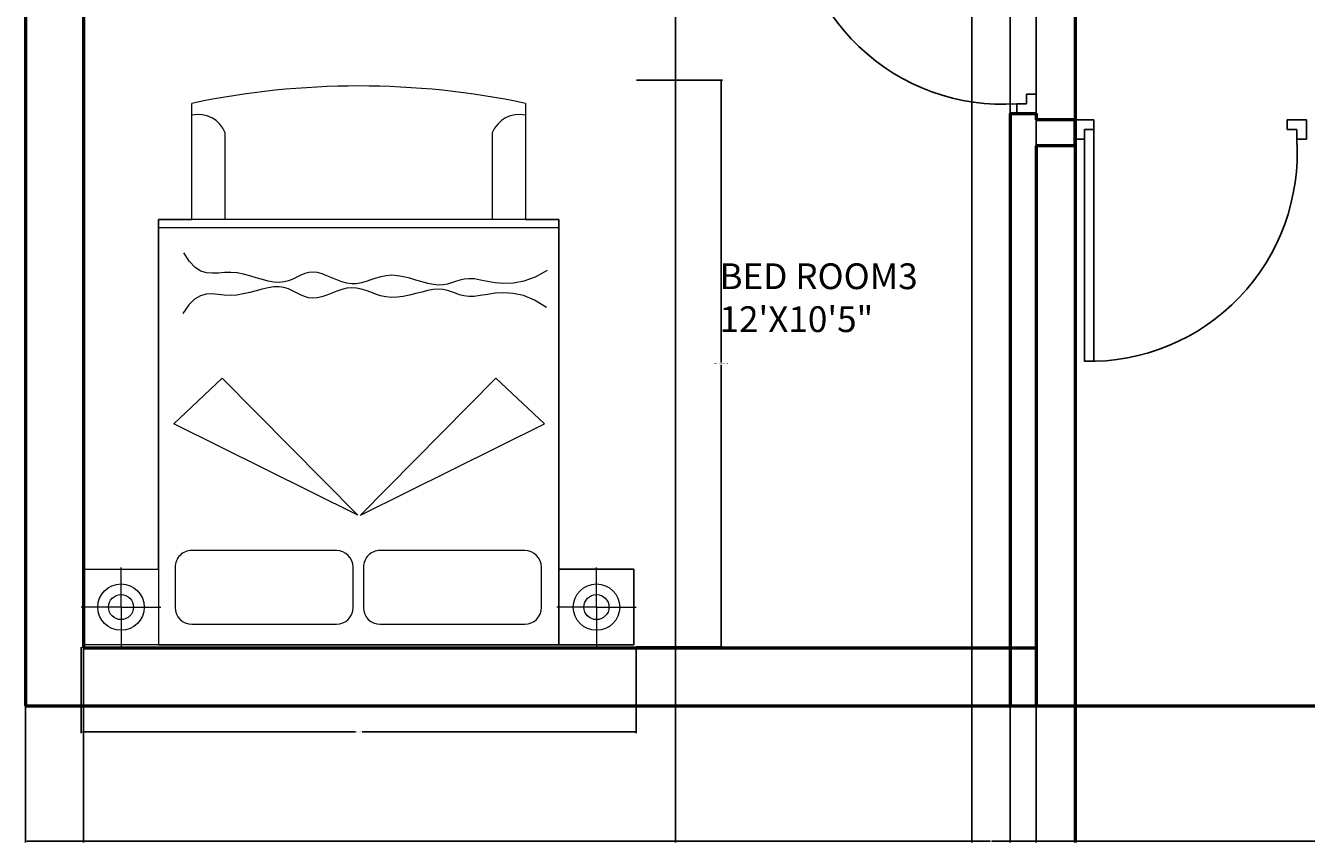
# Model space of a CAD drawing. Units: inches. Extents: x 1798 to 2141, y 1923 to 2386.
# Tile 1 of 9: x 1820 to 2019, y 1923 to 2050. Entities that reach past the tile are written whole.
import ezdxf

# ---------------------------------------------------------------- set-up
doc = ezdxf.new("R2010")
doc.units = ezdxf.units.IN
for name, color, linetype, lineweight in [('A-ANNO-DIMS', 2, 'Continuous', 18), ('A-AREA-IDEN', 7, 'Continuous', 25), ('A-FURN', 8, 'Continuous', 13), ('door', 40, 'Continuous', 25), ('wall', 4, 'Continuous', 50)]:
    doc.layers.add(name, color=color, linetype=linetype, lineweight=lineweight)
doc.styles.get("Standard").update_dxf_attribs({"font": 'arial.ttf'})
doc.dimstyles.get("Standard").update_dxf_attribs({"dimtxt": 0.18, "dimasz": 0.18, "dimexe": 0.18, "dimexo": 0.0625, "dimgap": 0.09, "dimtad": 0, "dimtih": 1, "dimtoh": 1, "dimdec": 4, "dimzin": 0, "dimdsep": 46, "dimtxsty": 'Standard', "dimcen": 0.09, "dimadec": 0, "dimazin": 0, "dimtfac": 1, "dimtdec": 4, "dimtofl": 0, "dimtmove": 0, "dimatfit": 3, "dimfxl": 1, "dimtolj": 1, "dimtzin": 0, "dimarcsym": 0})

# ---------------------------------------------------------------- blocks, each defined once
blk = doc.blocks.new('A$C4F543DC7')
for p, q in [((0.0134, 3.35, -0.1688), (3.3134, 3.35, -0.1688)), ((0.4634, 3.35, -0.1688), (0.0134, 3.35, -0.1688)), ((0.0134, 2.896, -0.1688), (0.0134, 3.35, -0.1688)), ((0.0134, 3.35, -0.1688), (0.0134, 2.896, -0.1688)), ((0.2381, 3.1233, -0.4388), (0.2381, 3.3614, -0.4388)), ((0.4634, 3.35, -0.1688), (0.4634, 0.8, -0.1688)), ((2.8634, 3.35, -0.1688), (0.4634, 3.35, -0.1688)), ((0.4634, 2.896, -0.1688), (0.4634, 3.35, -0.1688)), ((2.8634, 0.8, -0.1688), (2.8634, 3.35, -0.1688)), ((2.8634, 3.35, -0.1688), (3.3134, 3.35, -0.1688)), ((2.8634, 2.896, -0.1688), (2.8634, 3.35, -0.1688)), ((3.0888, 3.1233, -0.4388), (3.0888, 3.3614, -0.4388)), ((3.3134, 3.35, -0.1688), (3.3134, 2.896, -0.1688)), ((3.3134, 3.35, -0.1688), (3.3134, 2.896, -0.1688)), ((1.5354, 3.226, -0.1688), (0.6684, 3.226, -0.1688)), ((2.6644, 3.226, -0.1688), (1.7974, 3.226, -0.1688)), ((0.2381, 3.1233, -0.4388), (0, 3.1233, -0.4388)), ((0.2381, 3.1233, -0.4388), (0.4762, 3.1233, -0.4388)), ((0.2381, 3.1233, -0.4388), (0.2381, 2.8852, -0.4388)), ((0.5684, 3.126, -0.1688), (0.5684, 2.884, -0.1688)), ((1.6354, 2.884, -0.1688), (1.6354, 3.126, -0.1688)), ((1.6974, 3.126, -0.1688), (1.6974, 2.884, -0.1688)), ((2.7644, 2.884, -0.1688), (2.7644, 3.126, -0.1688)), ((3.0888, 3.1233, -0.4388), (2.8507, 3.1233, -0.4388)), ((3.0888, 3.1233, -0.4388), (3.0888, 2.8852, -0.4388)), ((3.0888, 3.1233, -0.4388), (3.3269, 3.1233, -0.4388)), ((0.4634, 2.896, -0.1688), (0.0134, 2.896, -0.1688)), ((0.0134, 2.896, -0.1688), (0.4634, 2.896, -0.1688)), ((0.4634, 0.8, -0.1688), (0.4634, 2.896, -0.1688)), ((2.8634, 2.896, -0.1688), (2.8634, 0.8, -0.1688)), ((3.3134, 2.896, -0.1688), (2.8634, 2.896, -0.1688)), ((3.3134, 2.896, -0.1688), (2.8634, 2.896, -0.1688)), ((0.6684, 2.784, -0.1688), (1.5354, 2.784, -0.1688)), ((1.7974, 2.784, -0.1688), (2.6644, 2.784, -0.1688)), ((1.6534, 2.573, -0.1688), (0.5504, 2.025, -0.1688)), ((0.8414, 1.752, -0.1688), (1.6534, 2.573, -0.1688)), ((2.4814, 1.752, -0.1688), (1.6694, 2.573, -0.1688)), ((1.6694, 2.573, -0.1688), (2.7724, 2.025, -0.1688)), ((0.5504, 2.025, -0.1688), (0.8414, 1.752, -0.1688)), ((2.7724, 2.025, -0.1688), (2.4814, 1.752, -0.1688)), ((0.5369, 1.3267, -0.1688), (0.6088, 1.2835, -0.1688)), ((2.6479, 1.2774, -0.1688), (2.683, 1.312, -0.1688)), ((2.683, 1.312, -0.1688), (2.7182, 1.3641, -0.1688)), ((0.6088, 1.2835, -0.1688), (0.6756, 1.2566, -0.1688)), ((0.6756, 1.2566, -0.1688), (0.7373, 1.2428, -0.1688)), ((0.7373, 1.2428, -0.1688), (0.794, 1.239, -0.1688)), ((0.794, 1.239, -0.1688), (0.8457, 1.242, -0.1688)), ((0.8457, 1.242, -0.1688), (0.8925, 1.2489, -0.1688)), ((0.8925, 1.2489, -0.1688), (0.9345, 1.2564, -0.1688)), ((0.9345, 1.2564, -0.1688), (0.9718, 1.2615, -0.1688)), ((0.9718, 1.2615, -0.1688), (1.0044, 1.2617, -0.1688)), ((1.0044, 1.2617, -0.1688), (1.0334, 1.2578, -0.1688)), ((1.0334, 1.2578, -0.1688), (1.0597, 1.2509, -0.1688)), ((1.0597, 1.2509, -0.1688), (1.0842, 1.2424, -0.1688)), ((1.0842, 1.2424, -0.1688), (1.1081, 1.2336, -0.1688)), ((1.1081, 1.2336, -0.1688), (1.1322, 1.2257, -0.1688)), ((1.2498, 1.2264, -0.1688), (1.2852, 1.2347, -0.1688)), ((1.2852, 1.2347, -0.1688), (1.3218, 1.2441, -0.1688)), ((1.3218, 1.2441, -0.1688), (1.3591, 1.2533, -0.1688)), ((1.3591, 1.2533, -0.1688), (1.3963, 1.2612, -0.1688)), ((1.3963, 1.2612, -0.1688), (1.4328, 1.2664, -0.1688)), ((1.4328, 1.2664, -0.1688), (1.4679, 1.2677, -0.1688)), ((1.4679, 1.2677, -0.1688), (1.501, 1.2643, -0.1688)), ((1.501, 1.2643, -0.1688), (1.5324, 1.257, -0.1688)), ((1.5324, 1.257, -0.1688), (1.5624, 1.2473, -0.1688)), ((1.5624, 1.2473, -0.1688), (1.5915, 1.2365, -0.1688)), ((1.5915, 1.2365, -0.1688), (1.6199, 1.2259, -0.1688)), ((1.7651, 1.2199, -0.1688), (1.7955, 1.2301, -0.1688)), ((1.7955, 1.2301, -0.1688), (1.8258, 1.2417, -0.1688)), ((1.8258, 1.2417, -0.1688), (1.8557, 1.2531, -0.1688)), ((1.8557, 1.2531, -0.1688), (1.8849, 1.263, -0.1688)), ((1.8849, 1.263, -0.1688), (1.913, 1.2698, -0.1688)), ((1.913, 1.2698, -0.1688), (1.9397, 1.2722, -0.1688)), ((1.9397, 1.2722, -0.1688), (1.9649, 1.2692, -0.1688)), ((1.9649, 1.2692, -0.1688), (1.989, 1.2617, -0.1688)), ((1.989, 1.2617, -0.1688), (2.0124, 1.2512, -0.1688)), ((2.0124, 1.2512, -0.1688), (2.0359, 1.2391, -0.1688)), ((2.0359, 1.2391, -0.1688), (2.0599, 1.2269, -0.1688)), ((2.2791, 1.2279, -0.1688), (2.3173, 1.2378, -0.1688)), ((2.3173, 1.2378, -0.1688), (2.3558, 1.2465, -0.1688)), ((2.3558, 1.2465, -0.1688), (2.3944, 1.2527, -0.1688)), ((2.3944, 1.2527, -0.1688), (2.4325, 1.255, -0.1688)), ((2.4325, 1.255, -0.1688), (2.4698, 1.2529, -0.1688)), ((2.4698, 1.2529, -0.1688), (2.5064, 1.2488, -0.1688)), ((2.5064, 1.2488, -0.1688), (2.5423, 1.2459, -0.1688)), ((2.5423, 1.2459, -0.1688), (2.5777, 1.2476, -0.1688)), ((2.5777, 1.2476, -0.1688), (2.6129, 1.257, -0.1688)), ((2.6129, 1.257, -0.1688), (2.6479, 1.2774, -0.1688)), ((0.6067, 1.1458, -0.1688), (0.6743, 1.1706, -0.1688)), ((0.6743, 1.1706, -0.1688), (0.7364, 1.1825, -0.1688)), ((0.7364, 1.1825, -0.1688), (0.7931, 1.1846, -0.1688)), ((0.7931, 1.1846, -0.1688), (0.8447, 1.1799, -0.1688)), ((0.8447, 1.1799, -0.1688), (0.8913, 1.1716, -0.1688)), ((0.8913, 1.1716, -0.1688), (0.9331, 1.1628, -0.1688)), ((0.9331, 1.1628, -0.1688), (0.9701, 1.1565, -0.1688)), ((0.9701, 1.1565, -0.1688), (1.0027, 1.1552, -0.1688)), ((1.0027, 1.1552, -0.1688), (1.0318, 1.1582, -0.1688)), ((1.0318, 1.1582, -0.1688), (1.0583, 1.1642, -0.1688)), ((1.0583, 1.1642, -0.1688), (1.0831, 1.172, -0.1688)), ((1.0831, 1.172, -0.1688), (1.1072, 1.18, -0.1688)), ((1.1072, 1.18, -0.1688), (1.1316, 1.1872, -0.1688)), ((1.1316, 1.1872, -0.1688), (1.1573, 1.192, -0.1688)), ((1.1322, 1.2257, -0.1688), (1.1577, 1.2201, -0.1688)), ((1.1573, 1.192, -0.1688), (1.1851, 1.1932, -0.1688)), ((1.1577, 1.2201, -0.1688), (1.1855, 1.218, -0.1688)), ((1.1851, 1.1932, -0.1688), (1.2158, 1.1898, -0.1688)), ((1.1855, 1.218, -0.1688), (1.2163, 1.2204, -0.1688)), ((1.2158, 1.1898, -0.1688), (1.2491, 1.1828, -0.1688)), ((1.2163, 1.2204, -0.1688), (1.2498, 1.2264, -0.1688)), ((1.2491, 1.1828, -0.1688), (1.2842, 1.1734, -0.1688)), ((1.2842, 1.1734, -0.1688), (1.3206, 1.1629, -0.1688)), ((1.3206, 1.1629, -0.1688), (1.3575, 1.1524, -0.1688)), ((1.3575, 1.1524, -0.1688), (1.3945, 1.1434, -0.1688)), ((1.5306, 1.1433, -0.1688), (1.5609, 1.152, -0.1688)), ((1.5609, 1.152, -0.1688), (1.5903, 1.1619, -0.1688)), ((1.5903, 1.1619, -0.1688), (1.6191, 1.1716, -0.1688)), ((1.6191, 1.1716, -0.1688), (1.6475, 1.1797, -0.1688)), ((1.6199, 1.2259, -0.1688), (1.6481, 1.2169, -0.1688)), ((1.6475, 1.1797, -0.1688), (1.676, 1.1849, -0.1688)), ((1.6481, 1.2169, -0.1688), (1.6765, 1.2108, -0.1688)), ((1.676, 1.1849, -0.1688), (1.7049, 1.1858, -0.1688)), ((1.6765, 1.2108, -0.1688), (1.7053, 1.209, -0.1688)), ((1.7049, 1.1858, -0.1688), (1.7344, 1.1816, -0.1688)), ((1.7053, 1.209, -0.1688), (1.7349, 1.2124, -0.1688)), ((1.7344, 1.1816, -0.1688), (1.7643, 1.1731, -0.1688)), ((1.7349, 1.2124, -0.1688), (1.7651, 1.2199, -0.1688)), ((1.7643, 1.1731, -0.1688), (1.7944, 1.1619, -0.1688)), ((1.7944, 1.1619, -0.1688), (1.8244, 1.1494, -0.1688)), ((2.0344, 1.1454, -0.1688), (2.0588, 1.1568, -0.1688)), ((2.0588, 1.1568, -0.1688), (2.0842, 1.167, -0.1688)), ((2.0599, 1.2269, -0.1688), (2.0849, 1.216, -0.1688)), ((2.0842, 1.167, -0.1688), (2.1112, 1.1743, -0.1688)), ((2.0849, 1.216, -0.1688), (2.1117, 1.2077, -0.1688)), ((2.1112, 1.1743, -0.1688), (2.1403, 1.1775, -0.1688)), ((2.1117, 1.2077, -0.1688), (2.1407, 1.2037, -0.1688)), ((2.1403, 1.1775, -0.1688), (2.1718, 1.1755, -0.1688)), ((2.1407, 1.2037, -0.1688), (2.1723, 1.2047, -0.1688)), ((2.1718, 1.1755, -0.1688), (2.2056, 1.1691, -0.1688)), ((2.1723, 1.2047, -0.1688), (2.2062, 1.21, -0.1688)), ((2.2056, 1.1691, -0.1688), (2.2411, 1.1598, -0.1688)), ((2.2062, 1.21, -0.1688), (2.242, 1.2182, -0.1688)), ((2.2411, 1.1598, -0.1688), (2.2779, 1.1489, -0.1688)), ((2.242, 1.2182, -0.1688), (2.2791, 1.2279, -0.1688)), ((0.5334, 1.105, -0.1688), (0.6067, 1.1458, -0.1688)), ((1.3945, 1.1434, -0.1688), (1.4308, 1.1371, -0.1688)), ((1.4308, 1.1371, -0.1688), (1.4658, 1.1347, -0.1688)), ((1.4658, 1.1347, -0.1688), (1.499, 1.137, -0.1688)), ((1.499, 1.137, -0.1688), (1.5306, 1.1433, -0.1688)), ((1.8244, 1.1494, -0.1688), (1.8539, 1.137, -0.1688)), ((1.8539, 1.137, -0.1688), (1.8827, 1.1263, -0.1688)), ((1.8827, 1.1263, -0.1688), (1.9106, 1.1186, -0.1688)), ((1.9106, 1.1186, -0.1688), (1.9373, 1.1153, -0.1688)), ((1.9373, 1.1153, -0.1688), (1.9625, 1.1176, -0.1688)), ((1.9625, 1.1176, -0.1688), (1.9868, 1.1243, -0.1688)), ((1.9868, 1.1243, -0.1688), (2.0106, 1.134, -0.1688)), ((2.0106, 1.134, -0.1688), (2.0344, 1.1454, -0.1688)), ((2.2779, 1.1489, -0.1688), (2.3157, 1.1379, -0.1688)), ((2.3157, 1.1379, -0.1688), (2.354, 1.1279, -0.1688)), ((2.354, 1.1279, -0.1688), (2.3923, 1.1205, -0.1688)), ((2.3923, 1.1205, -0.1688), (2.4304, 1.117, -0.1688)), ((2.4304, 1.117, -0.1688), (2.4677, 1.118, -0.1688)), ((2.4677, 1.118, -0.1688), (2.5043, 1.1209, -0.1688)), ((2.5043, 1.1209, -0.1688), (2.5403, 1.1226, -0.1688)), ((2.5403, 1.1226, -0.1688), (2.5757, 1.1199, -0.1688)), ((2.5757, 1.1199, -0.1688), (2.6106, 1.1094, -0.1688)), ((2.6106, 1.1094, -0.1688), (2.645, 1.0879, -0.1688)), ((2.645, 1.0879, -0.1688), (2.6789, 1.0522, -0.1688)), ((2.6789, 1.0522, -0.1688), (2.7124, 0.999, -0.1688)), ((0.4634, 0.85, -0.1688), (2.8634, 0.85, -0.1688)), ((0.4634, 0.8, -0.1688), (2.8634, 0.8, -0.1688)), ((0.6634, 0.8, -0.1688), (0.4634, 0.8, -0.1688)), ((0.6634, 0.8, -0.1688), (2.6634, 0.8, -0.1688)), ((0.6634, 0.104, -0.1688), (0.6634, 0.8, -0.1688)), ((0.6634, 0.104, -0.1688), (0.6634, 0.8, -0.1688)), ((0.8634, 0.281, -0.1688), (0.8634, 0.8, -0.1688)), ((2.4634, 0.8, -0.1688), (2.4634, 0.281, -0.1688)), ((2.8634, 0.8, -0.1688), (2.6634, 0.8, -0.1688)), ((2.6634, 0.8, -0.1688), (2.6634, 0.104, -0.1688)), ((2.6634, 0.8, -0.1688), (2.6634, 0.104, -0.1688))]:
    blk.add_line(p, q)
for centre, radius in [((0.2381, 3.1233, -0.4388), 0.139), ((3.0888, 3.1233, -0.4388), 0.139), ((0.2381, 3.1233, -0.4388), 0.075), ((3.0888, 3.1233, -0.4388), 0.075)]:
    blk.add_circle(centre, radius)
for centre, radius, start, end in [((0.6684, 3.126, -0.1688), 0.1, 90, 180), ((1.5354, 3.126, -0.1688), 0.1, 0, 90), ((1.7974, 3.126, -0.1688), 0.1, 90, 180), ((2.6644, 3.126, -0.1688), 0.1, 0, 90), ((0.6684, 2.884, -0.1688), 0.1, 180, 270), ((1.5354, 2.884, -0.1688), 0.1, 270, 0), ((1.7974, 2.884, -0.1688), 0.1, 180, 270), ((2.6644, 2.884, -0.1688), 0.1, 270, 0), ((0.6994, 0.3472, -0.1688), 0.1769, 258.2616, 338.03196), ((2.6275, 0.3472, -0.1688), 0.1769, 201.96804, 281.7384), ((1.6634, 4.8597, -0.1688), 4.8597, 258.12517, 281.87483), ((1.6634, 4.8597, -0.1688), 4.8597, 258.12517, 281.87483)]:
    blk.add_arc(centre, radius, start, end)
blk = doc.blocks.new('DOOR-SWING-36IN')
for p, q in [((1.5, 1.5), (1.5, 37.5)), ((3, 1.5), (3, 37.5)), ((0, 3), (0, 0)), ((1.5, 3), (0, 3)), ((1.5, 1.5), (1.5, 3)), ((34.5, 1.5), (34.5, 3)), ((34.5, 3), (36, 3)), ((36, 3), (36, 0)), ((3, 1.5), (1.5, 1.5)), ((3, 0), (3, 1.5)), ((33, 0), (33, 1.5)), ((33, 1.5), (34.5, 1.5)), ((0, 0), (3, 0)), ((36, 0), (33, 0))]:
    blk.add_line(p, q)
blk.add_arc((2.25, 5.18), 32.32, 356.1244, 91.3295)
blk = doc.blocks.new('*D17')
at = {"layer": 'A-ANNO-DIMS', "color": 0, "lineweight": -2, "transparency": 16777216}
for p, q in [((1914.45, 2041.5), (1927.77, 2041.5)), ((1927.59, 2041.32), (1927.59, 1997.67)), ((1927.59, 1953.67), (1927.59, 1997.31)), ((1914.45, 1953.49), (1927.77, 1953.49))]:
    blk.add_line(p, q, dxfattribs=at)
at = {"layer": 'A-ANNO-DIMS', "color": 0, "transparency": 16777216}
for points in [[(1927.56, 2041.32), (1927.62, 2041.32), (1927.59, 2041.5)], [(1927.56, 1953.67), (1927.62, 1953.67), (1927.59, 1953.49)]]:
    blk.add_solid(points, dxfattribs=at)
at = {"layer": 'Defpoints', "color": 0, "transparency": 16777216}
for p in [(1914.38, 2041.5), (1914.38, 1953.49), (1927.59, 1953.49)]:
    blk.add_point(p, dxfattribs=at)
at = {"layer": 'A-ANNO-DIMS', "color": 0, "transparency": 16777216, "insert": (1927.59, 1997.49), "char_height": 0.18, "attachment_point": 5}
blk.add_mtext('\\A1;BED GROUP 88 TYP.', dxfattribs=at)
blk = doc.blocks.new('*D18')
at = {"layer": 'A-ANNO-DIMS', "color": 0, "lineweight": -2, "transparency": 16777216}
for p, q in [((1828.17, 1953.42), (1828.17, 1940.1)), ((1914.38, 1953.42), (1914.38, 1940.1)), ((1828.35, 1940.28), (1870.75, 1940.28)), ((1914.2, 1940.28), (1871.8, 1940.28))]:
    blk.add_line(p, q, dxfattribs=at)
at = {"layer": 'A-ANNO-DIMS', "color": 0, "transparency": 16777216}
for points in [[(1828.35, 1940.31), (1828.35, 1940.25), (1828.17, 1940.28)], [(1914.2, 1940.31), (1914.2, 1940.25), (1914.38, 1940.28)]]:
    blk.add_solid(points, dxfattribs=at)
at = {"layer": 'Defpoints', "color": 0, "transparency": 16777216}
for p in [(1828.17, 1953.49), (1914.38, 1953.49), (1828.17, 1940.28)]:
    blk.add_point(p, dxfattribs=at)
at = {"layer": 'A-ANNO-DIMS', "color": 0, "transparency": 16777216, "insert": (1871.27, 1940.28), "char_height": 0.18, "attachment_point": 5}
blk.add_mtext('\\A1;86 TYP.', dxfattribs=at)
blk = doc.blocks.new('*D31')
at = {"layer": 'A-ANNO-DIMS', "color": 0, "lineweight": -2, "transparency": 16777216}
for p, q in [((1819.51, 1944.26), (1819.51, 1923.12)), ((2119.51, 1944.26), (2119.51, 1923.12)), ((1819.69, 1923.3), (1969.23, 1923.3)), ((2119.33, 1923.3), (1969.8, 1923.3))]:
    blk.add_line(p, q, dxfattribs=at)
at = {"layer": 'A-ANNO-DIMS', "color": 0, "transparency": 16777216}
for points in [[(1819.69, 1923.33), (1819.69, 1923.27), (1819.51, 1923.3)], [(2119.33, 1923.33), (2119.33, 1923.27), (2119.51, 1923.3)]]:
    blk.add_solid(points, dxfattribs=at)
at = {"layer": 'Defpoints', "color": 0, "transparency": 16777216}
for p in [(1819.51, 1944.32), (2119.51, 1944.32), (2119.51, 1923.3)]:
    blk.add_point(p, dxfattribs=at)
at = {"layer": 'A-ANNO-DIMS', "color": 0, "transparency": 16777216, "insert": (1969.51, 1923.3), "char_height": 0.18, "attachment_point": 5}
blk.add_mtext('\\A1;300', dxfattribs=at)
blk = doc.blocks.new('*D35')
at = {"layer": 'A-ANNO-DIMS', "color": 0, "lineweight": -2, "transparency": 16777216}
for p, q in [((1972.51, 2235.26), (1972.51, 1923.12)), ((1966.51, 2231.26), (1966.51, 1923.12)), ((1966.69, 1923.3), (1969.36, 1923.3)), ((1972.33, 1923.3), (1969.66, 1923.3))]:
    blk.add_line(p, q, dxfattribs=at)
at = {"layer": 'A-ANNO-DIMS', "color": 0, "transparency": 16777216}
for points in [[(1966.69, 1923.33), (1966.69, 1923.27), (1966.51, 1923.3)], [(1972.33, 1923.33), (1972.33, 1923.27), (1972.51, 1923.3)]]:
    blk.add_solid(points, dxfattribs=at)
at = {"layer": 'Defpoints', "color": 0, "transparency": 16777216}
for p in [(1972.51, 2235.32), (1966.51, 2231.32), (1972.51, 1923.3)]:
    blk.add_point(p, dxfattribs=at)
at = {"layer": 'A-ANNO-DIMS', "color": 0, "transparency": 16777216, "insert": (1969.51, 1923.3), "char_height": 0.18, "attachment_point": 5}
blk.add_mtext('\\A1;6', dxfattribs=at)
blk = doc.blocks.new('*D36')
at = {"layer": 'A-ANNO-DIMS', "color": 0, "lineweight": -2, "transparency": 16777216}
for p, q in [((1976.51, 2231.26), (1976.51, 1923.12)), ((1982.51, 2231.26), (1982.51, 1923.12)), ((1976.69, 1923.3), (1979.36, 1923.3)), ((1982.33, 1923.3), (1979.66, 1923.3))]:
    blk.add_line(p, q, dxfattribs=at)
at = {"layer": 'A-ANNO-DIMS', "color": 0, "transparency": 16777216}
for points in [[(1976.69, 1923.33), (1976.69, 1923.27), (1976.51, 1923.3)], [(1982.33, 1923.33), (1982.33, 1923.27), (1982.51, 1923.3)]]:
    blk.add_solid(points, dxfattribs=at)
at = {"layer": 'Defpoints', "color": 0, "transparency": 16777216}
for p in [(1976.51, 2231.32), (1982.51, 2231.32), (1982.51, 1923.3)]:
    blk.add_point(p, dxfattribs=at)
at = {"layer": 'A-ANNO-DIMS', "color": 0, "transparency": 16777216, "insert": (1979.51, 1923.3), "char_height": 0.18, "attachment_point": 5}
blk.add_mtext('\\A1;6', dxfattribs=at)
blk = doc.blocks.new('*D39')
at = {"layer": 'A-ANNO-DIMS', "color": 0, "lineweight": -2, "transparency": 16777216}
for p, q in [((1976.51, 2035.39), (1976.51, 2385.53)), ((1976.69, 2385.35), (1979.36, 2385.35)), ((1982.33, 2385.35), (1979.66, 2385.35)), ((1982.51, 2035.39), (1982.51, 2385.53))]:
    blk.add_line(p, q, dxfattribs=at)
at = {"layer": 'A-ANNO-DIMS', "color": 0, "transparency": 16777216}
for points in [[(1976.69, 2385.38), (1976.69, 2385.32), (1976.51, 2385.35)], [(1982.33, 2385.38), (1982.33, 2385.32), (1982.51, 2385.35)]]:
    blk.add_solid(points, dxfattribs=at)
at = {"layer": 'Defpoints', "color": 0, "transparency": 16777216}
for p in [(1982.51, 2385.35), (1976.51, 2035.32), (1982.51, 2035.32)]:
    blk.add_point(p, dxfattribs=at)
at = {"layer": 'A-ANNO-DIMS', "color": 0, "transparency": 16777216, "insert": (1979.51, 2385.35), "char_height": 0.18, "attachment_point": 5}
blk.add_mtext('\\A1;6', dxfattribs=at)
blk = doc.blocks.new('*D41')
at = {"layer": 'A-ANNO-DIMS', "color": 0, "lineweight": -2, "transparency": 16777216}
for p, q in [((1828.51, 2082.26), (1828.51, 1923.12)), ((1920.51, 2082.26), (1920.51, 1923.12)), ((1828.69, 1923.3), (1874.3, 1923.3)), ((1920.33, 1923.3), (1874.73, 1923.3))]:
    blk.add_line(p, q, dxfattribs=at)
at = {"layer": 'A-ANNO-DIMS', "color": 0, "transparency": 16777216}
for points in [[(1828.69, 1923.33), (1828.69, 1923.27), (1828.51, 1923.3)], [(1920.33, 1923.33), (1920.33, 1923.27), (1920.51, 1923.3)]]:
    blk.add_solid(points, dxfattribs=at)
at = {"layer": 'Defpoints', "color": 0, "transparency": 16777216}
for p in [(1828.51, 2082.32), (1920.51, 2082.32), (1920.51, 1923.3)]:
    blk.add_point(p, dxfattribs=at)
at = {"layer": 'A-ANNO-DIMS', "color": 0, "transparency": 16777216, "insert": (1874.51, 1923.3), "char_height": 0.18, "attachment_point": 5}
blk.add_mtext('\\A1;92', dxfattribs=at)
blk = doc.blocks.new('*D46')
at = {"layer": 'A-ANNO-DIMS', "color": 0, "lineweight": -2, "transparency": 16777216}
for p, q in [((1982.72, 2148.29), (1982.72, 1923.12)), ((2034.51, 2135.26), (2034.51, 1923.12)), ((1982.9, 1923.3), (2008.22, 1923.3)), ((2034.33, 1923.3), (2009.01, 1923.3))]:
    blk.add_line(p, q, dxfattribs=at)
at = {"layer": 'A-ANNO-DIMS', "color": 0, "transparency": 16777216}
for points in [[(1982.9, 1923.33), (1982.9, 1923.27), (1982.72, 1923.3)], [(2034.33, 1923.33), (2034.33, 1923.27), (2034.51, 1923.3)]]:
    blk.add_solid(points, dxfattribs=at)
at = {"layer": 'Defpoints', "color": 0, "transparency": 16777216}
for p in [(1982.72, 2148.35), (2034.51, 2135.32), (2034.51, 1923.3)]:
    blk.add_point(p, dxfattribs=at)
at = {"layer": 'A-ANNO-DIMS', "color": 0, "transparency": 16777216, "insert": (2008.62, 1923.3), "char_height": 0.18, "attachment_point": 5}
blk.add_mtext('\\A1;51.79', dxfattribs=at)

msp = doc.modelspace()

# ---------------------------------------------------------------- linework, layer by layer
at = {"layer": 'wall'}
for p, q in [((1819.5141, 2364.3239), (1819.5141, 1944.3239)), ((1828.5141, 2355.3239), (1828.5141, 1953.3239)), ((1972.5141, 2036.3239), (1976.5141, 2036.3239)), ((1972.5141, 2036.3239), (1972.5141, 1944.3239)), ((1976.5141, 2036.3239), (1976.5141, 2035.3239)), ((1982.5141, 2035.3239), (1976.5141, 2035.3239)), ((1982.5141, 2035.3239), (1982.5141, 2031.3239)), ((1976.5141, 2031.3239), (1976.5141, 1944.3239)), ((1982.5141, 2031.3239), (1976.5141, 2031.3239)), ((1828.5141, 1953.3239), (1976.5141, 1953.3239)), ((1819.5141, 1944.3239), (2119.5141, 1944.3239))]:
    msp.add_line(p, q, dxfattribs=at)

# ---------------------------------------------------------------- block references
at = {"layer": 'A-FURN', "xscale": 25.91562772622874, "yscale": 25.91562772622874, "zscale": 25.91562772622874, "rotation": 180}
msp.add_blockref('A$C4F543DC7', (1914.3839, 2040.5975, 4.3733), dxfattribs=at)
at = {"layer": 'door', "extrusion": (0, 0, -1), "zscale": -1}
for p, rotation in [((-1976.5141, 2072.3239), 269.9999999999993), ((-1982.5141, 2035.3239), 180)]:
    msp.add_blockref('DOOR-SWING-36IN', p, dxfattribs=dict(at, rotation=rotation))

# ---------------------------------------------------------------- texts
at = {"layer": 'A-AREA-IDEN', "insert": (1927.3263, 2013.0466), "char_height": 4, "attachment_point": 1}
msp.add_mtext_dynamic_manual_height_columns('\\pxt7;BED ROOM3\\P12\'X10\'5"', width=37.733578, gutter_width=12.5, heights=[21.4385], dxfattribs=at)

# ---------------------------------------------------------------- dimensions: what is measured, and where the dimension line sits
at = {"layer": 'A-ANNO-DIMS'}
for base, p1, p2, override, picture, middle in [((1982.5141, 2385.3489), (1976.5141, 2035.3239), (1982.5141, 2035.3239), {"dimdec": 0, "dimlfac": 1, "dimrnd": 0, "dimzin": 0, "dimdsep": 46, "dimlunit": 2}, '*D39', (1979.5141, 2385.3489)), ((1972.5141, 1923.2989), (1966.5141, 2231.3239), (1972.5141, 2235.3239), {"dimdec": 0, "dimlfac": 1, "dimrnd": 0, "dimzin": 0, "dimdsep": 46, "dimlunit": 2}, '*D35', (1969.5141, 1923.2989)), ((1982.5141, 1923.2989), (1976.5141, 2231.3239), (1982.5141, 2231.3239), {"dimdec": 0, "dimlfac": 1, "dimrnd": 0, "dimzin": 0, "dimdsep": 46, "dimlunit": 2}, '*D36', (1979.5141, 1923.2989)), ((2034.5141, 1923.2989), (1982.7222, 2148.3502), (2034.5141, 2135.3239), {"dimdec": 2, "dimlfac": 1, "dimrnd": 0, "dimzin": 0, "dimdsep": 46, "dimlunit": 2}, '*D46', (2008.6182, 1923.2989)), ((1920.5141, 1923.2989), (1828.5141, 2082.3239), (1920.5141, 2082.3239), {"dimdec": 0, "dimlfac": 1, "dimrnd": 0, "dimzin": 0, "dimdsep": 46, "dimlunit": 2}, '*D41', (1874.5141, 1923.2989)), ((2119.5141, 1923.2989), (1819.5141, 1944.3239), (2119.5141, 1944.3239), {"dimdec": 0, "dimlfac": 1, "dimrnd": 0, "dimzin": 0, "dimdsep": 46, "dimlunit": 2}, '*D31', (1969.5141, 1923.2989))]:
    dim = msp.add_linear_dim(base=base, p1=p1, p2=p2, dimstyle='Standard', override=override, dxfattribs=at)
    dim.commit()
    dim.dimension.update_dxf_attribs({"geometry": picture, "text_midpoint": middle})
for base, p1, p2, angle, text, picture, middle in [((1927.5855, 1953.4853), (1914.3839, 2041.4959), (1914.3839, 1953.4853), 270, 'BED GROUP <> TYP.', '*D17', (1927.5855, 1997.4906)), ((1828.1659, 1940.2837), (1914.3839, 1953.4853), (1828.1659, 1953.4853), 180, '<> TYP.', '*D18', (1871.2749, 1940.2837))]:
    dim = msp.add_linear_dim(base=base, p1=p1, p2=p2, angle=angle, text=text, dimstyle='Standard', override={"dimdec": 0, "dimlfac": 1, "dimrnd": 0, "dimzin": 0, "dimdsep": 46, "dimlunit": 2}, dxfattribs=at)
    dim.commit()
    dim.dimension.update_dxf_attribs({"geometry": picture, "text_midpoint": middle})

doc.saveas('drawing.dxf')
